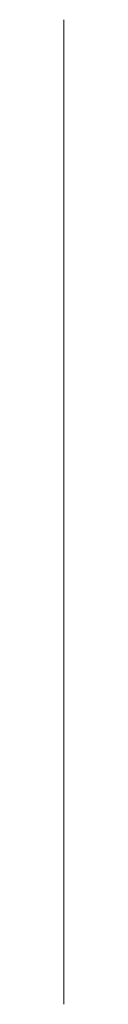
# Model space of a CAD drawing. Units: millimetres. Extents: x -182.5 to -182.5, y 315.3 to 372.3.
import ezdxf

# ---------------------------------------------------------------- set-up
doc = ezdxf.new("R2010")
doc.units = ezdxf.units.MM
doc.layers.add('M-CONS', color=8, linetype='Continuous', lineweight=13)

msp = doc.modelspace()

# ---------------------------------------------------------------- linework, layer by layer
at = {"layer": 'M-CONS'}
msp.add_line((-182.537, 372.318, 354.457), (-182.537, 315.318, 354.457), dxfattribs=at)

doc.saveas('drawing.dxf')
